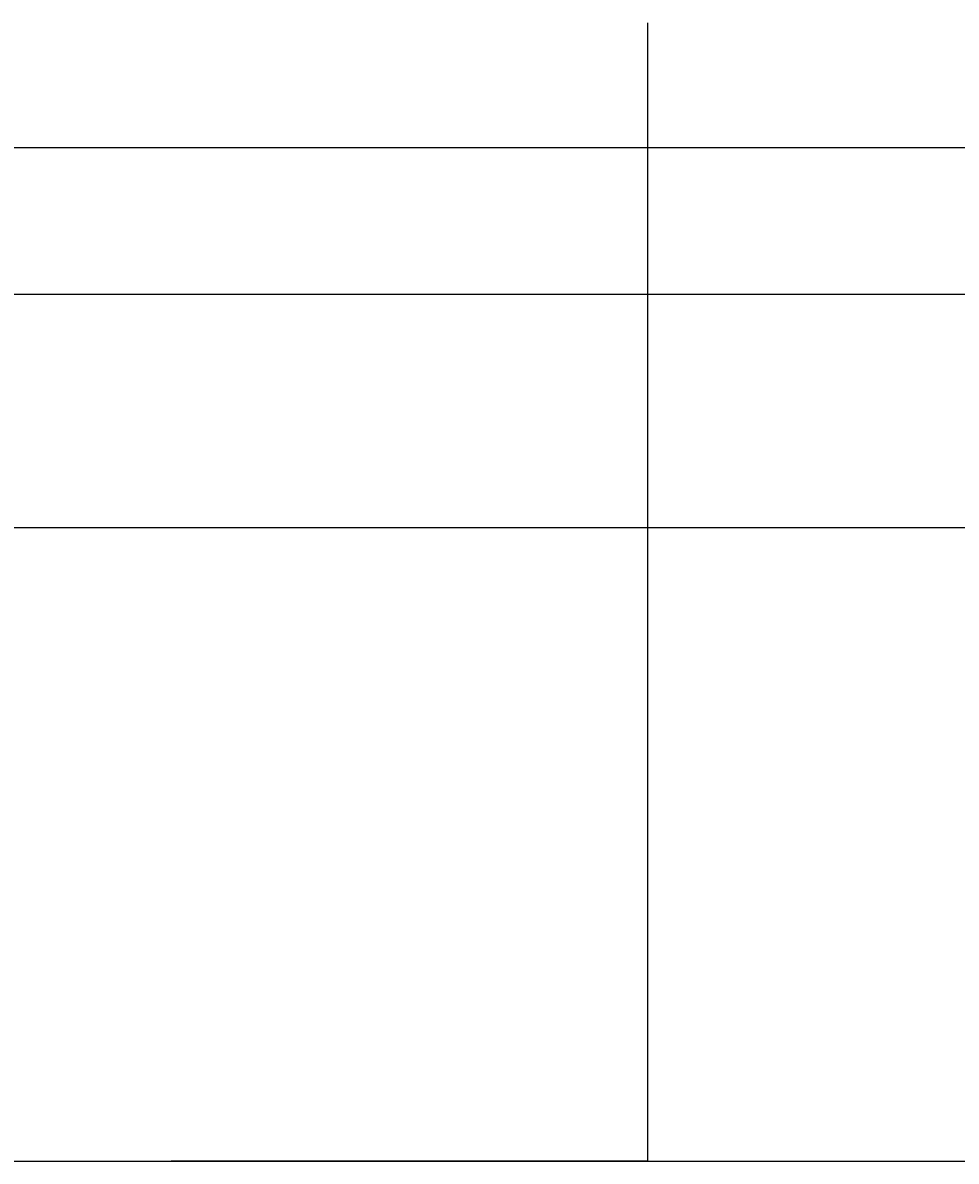
# Model space of a CAD drawing. Units: inches. Extents: x 35362 to 73946, y 43607 to 67532.
# Tile 2 of 134: x 38077 to 40793, y 43607 to 46919. Entities that reach past the tile are written whole.
import ezdxf

# ---------------------------------------------------------------- set-up
doc = ezdxf.new("R2010")
doc.units = ezdxf.units.IN
doc.header["$MEASUREMENT"] = 0
doc.layers.add('A-ANNO-DIMS', color=2, linetype='Continuous', lineweight=18)
doc.styles.get("Standard").update_dxf_attribs({"font": 'arial.ttf'})
doc.dimstyles.get("Standard").update_dxf_attribs({"dimtxt": 0.18, "dimasz": 0.18, "dimexe": 0.18, "dimexo": 0.0625, "dimgap": 0.09, "dimtad": 0, "dimtih": 1, "dimtoh": 1, "dimdec": 4, "dimzin": 0, "dimdsep": 46, "dimtxsty": 'Standard', "dimcen": 0.09, "dimadec": 0, "dimazin": 0, "dimtfac": 1, "dimtdec": 4, "dimtofl": 0, "dimtmove": 0, "dimatfit": 3, "dimfxl": 1, "dimtolj": 1, "dimtzin": 0, "dimarcsym": 0})

# ---------------------------------------------------------------- blocks, each defined once
blk = doc.blocks.new('*D5')
at = {"layer": 'A-ANNO-DIMS', "color": 0, "lineweight": -2, "transparency": 16777216}
for p, q in [((37121.9, 46919.3), (37121.9, 43606.7)), ((69871.5, 45449.8), (69871.5, 43606.7)), ((37122.1, 43606.9), (53496.3, 43606.9)), ((69871.3, 43606.9), (53497.2, 43606.9))]:
    blk.add_line(p, q, dxfattribs=at)
at = {"layer": 'A-ANNO-DIMS', "color": 0, "transparency": 16777216}
for points in [[(37122.1, 43606.9), (37122.1, 43606.8), (37121.9, 43606.9)], [(69871.3, 43606.9), (69871.3, 43606.8), (69871.5, 43606.9)]]:
    blk.add_solid(points, dxfattribs=at)
at = {"layer": 'Defpoints', "color": 0, "transparency": 16777216}
for p in [(37121.9, 46919.4), (69871.5, 45449.9), (69871.5, 43606.9)]:
    blk.add_point(p, dxfattribs=at)
at = {"layer": 'A-ANNO-DIMS', "color": 0, "transparency": 16777216, "insert": (53496.7, 43606.9), "char_height": 0.18, "attachment_point": 5}
blk.add_mtext('\\A1;32750', dxfattribs=at)
blk = doc.blocks.new('*D15')
at = {"layer": 'A-ANNO-DIMS', "color": 0, "lineweight": -2, "transparency": 16777216}
for p, q in [((37121.9, 46919.3), (37121.9, 43606.7)), ((39894.8, 46919.3), (39894.8, 43606.7)), ((37122.1, 43606.9), (38508, 43606.9)), ((39894.7, 43606.9), (38508.8, 43606.9))]:
    blk.add_line(p, q, dxfattribs=at)
at = {"layer": 'A-ANNO-DIMS', "color": 0, "transparency": 16777216}
for points in [[(37122.1, 43606.9), (37122.1, 43606.8), (37121.9, 43606.9)], [(39894.7, 43606.9), (39894.7, 43606.8), (39894.8, 43606.9)]]:
    blk.add_solid(points, dxfattribs=at)
at = {"layer": 'Defpoints', "color": 0, "transparency": 16777216}
for p in [(37121.9, 46919.4), (39894.8, 46919.4), (39894.8, 43606.9)]:
    blk.add_point(p, dxfattribs=at)
at = {"layer": 'A-ANNO-DIMS', "color": 0, "transparency": 16777216, "insert": (38508.4, 43606.9), "char_height": 0.18, "attachment_point": 5}
blk.add_mtext('\\A1;2773', dxfattribs=at)
blk = doc.blocks.new('*D41')
at = {"layer": 'A-ANNO-DIMS', "color": 0, "lineweight": -2, "transparency": 16777216}
for p, q in [((39894.8, 46919.3), (39894.8, 43606.7)), ((45390.1, 46919.3), (45390.1, 43606.7)), ((39895, 43606.9), (42642, 43606.9)), ((45390, 43606.9), (42643, 43606.9))]:
    blk.add_line(p, q, dxfattribs=at)
at = {"layer": 'A-ANNO-DIMS', "color": 0, "transparency": 16777216}
for points in [[(39895, 43606.9), (39895, 43606.8), (39894.8, 43606.9)], [(45390, 43606.9), (45390, 43606.8), (45390.1, 43606.9)]]:
    blk.add_solid(points, dxfattribs=at)
at = {"layer": 'Defpoints', "color": 0, "transparency": 16777216}
for p in [(39894.8, 46919.4), (45390.1, 46919.4), (45390.1, 43606.9)]:
    blk.add_point(p, dxfattribs=at)
at = {"layer": 'A-ANNO-DIMS', "color": 0, "transparency": 16777216, "insert": (42642.5, 43606.9), "char_height": 0.18, "attachment_point": 5}
blk.add_mtext('\\A1;5495.3', dxfattribs=at)
blk = doc.blocks.new('*D67')
at = {"layer": 'A-ANNO-DIMS', "color": 0, "lineweight": -2, "transparency": 16777216}
for p, q in [((56873.5, 53351.5), (35361.8, 53351.5)), ((35361.9, 53351.3), (35361.9, 49400.9)), ((35361.9, 45450.1), (35361.9, 49400.5)), ((53793.6, 45449.9), (35361.8, 45449.9))]:
    blk.add_line(p, q, dxfattribs=at)
at = {"layer": 'A-ANNO-DIMS', "color": 0, "transparency": 16777216}
for points in [[(35361.9, 53351.3), (35362, 53351.3), (35361.9, 53351.5)], [(35361.9, 45450.1), (35362, 45450.1), (35361.9, 45449.9)]]:
    blk.add_solid(points, dxfattribs=at)
at = {"layer": 'Defpoints', "color": 0, "transparency": 16777216}
for p in [(35361.9, 53351.5), (56873.6, 53351.5), (53793.6, 45449.9)]:
    blk.add_point(p, dxfattribs=at)
at = {"layer": 'A-ANNO-DIMS', "color": 0, "transparency": 16777216, "insert": (35361.9, 49400.7), "char_height": 0.18, "attachment_point": 5}
blk.add_mtext('\\A1;7901.6', dxfattribs=at)
blk = doc.blocks.new('*D76')
at = {"layer": 'A-ANNO-DIMS', "color": 0, "lineweight": -2, "transparency": 16777216}
for p, q in [((54052.8, 46555.3), (35361.8, 46555.3)), ((35361.9, 46555.1), (35361.9, 46342.3)), ((35361.9, 46129.1), (35361.9, 46341.9)), ((53793.6, 46128.9), (35361.8, 46128.9))]:
    blk.add_line(p, q, dxfattribs=at)
at = {"layer": 'A-ANNO-DIMS', "color": 0, "transparency": 16777216}
for points in [[(35361.9, 46555.1), (35362, 46555.1), (35361.9, 46555.3)], [(35361.9, 46129.1), (35362, 46129.1), (35361.9, 46128.9)]]:
    blk.add_solid(points, dxfattribs=at)
at = {"layer": 'Defpoints', "color": 0, "transparency": 16777216}
for p in [(35361.9, 46555.3), (54052.9, 46555.3), (53793.6, 46128.9)]:
    blk.add_point(p, dxfattribs=at)
at = {"layer": 'A-ANNO-DIMS', "color": 0, "transparency": 16777216, "insert": (35361.9, 46342.1), "char_height": 0.18, "attachment_point": 5}
blk.add_mtext('\\A1;426.4', dxfattribs=at)
blk = doc.blocks.new('*D90')
at = {"layer": 'A-ANNO-DIMS', "color": 0, "lineweight": -2, "transparency": 16777216}
for p, q in [((53707.7, 47291.3), (35361.8, 47291.3)), ((35361.9, 47291.1), (35361.9, 46710.3)), ((35361.9, 46129.1), (35361.9, 46709.9)), ((53793.6, 46128.9), (35361.8, 46128.9))]:
    blk.add_line(p, q, dxfattribs=at)
at = {"layer": 'A-ANNO-DIMS', "color": 0, "transparency": 16777216}
for points in [[(35361.9, 47291.1), (35362, 47291.1), (35361.9, 47291.3)], [(35361.9, 46129.1), (35362, 46129.1), (35361.9, 46128.9)]]:
    blk.add_solid(points, dxfattribs=at)
at = {"layer": 'Defpoints', "color": 0, "transparency": 16777216}
for p in [(53707.8, 47291.3), (35361.9, 46128.9), (53793.6, 46128.9)]:
    blk.add_point(p, dxfattribs=at)
at = {"layer": 'A-ANNO-DIMS', "color": 0, "transparency": 16777216, "insert": (35361.9, 46710.1), "char_height": 0.18, "attachment_point": 5}
blk.add_mtext('\\A1;1162.4', dxfattribs=at)

msp = doc.modelspace()

# ---------------------------------------------------------------- dimensions: what is measured, and where the dimension line sits
at = {"layer": 'A-ANNO-DIMS'}
for base, p1, p2, picture, middle in [((35361.949, 53351.529), (53793.638, 45449.894), (56873.602, 53351.529), '*D67', (35361.949, 49400.712)), ((35361.949, 46128.878), (53707.781, 47291.285), (53793.638, 46128.878), '*D90', (35361.949, 46710.081)), ((35361.949, 46555.293), (53793.638, 46128.878), (54052.899, 46555.293), '*D76', (35361.949, 46342.086))]:
    dim = msp.add_linear_dim(base=base, p1=p1, p2=p2, angle=90, dimstyle='Standard', override={"dimdec": 1, "dimlfac": 1, "dimrnd": 0, "dimzin": 0, "dimdsep": 46, "dimlunit": 2}, dxfattribs=at)
    dim.commit()
    dim.dimension.update_dxf_attribs({"geometry": picture, "text_midpoint": middle})
for base, p1, p2, override, picture, middle in [((69871.496, 43606.859), (37121.949, 46919.381), (69871.496, 45449.894), {"dimdec": 0, "dimlfac": 1, "dimrnd": 0, "dimzin": 0, "dimdsep": 46, "dimlunit": 2}, '*D5', (53496.723, 43606.859)), ((39894.84, 43606.859), (37121.949, 46919.381), (39894.84, 46919.381), {"dimdec": 0, "dimlfac": 1, "dimrnd": 0, "dimzin": 0, "dimdsep": 46, "dimlunit": 2}, '*D15', (38508.395, 43606.859)), ((45390.147, 43606.859), (39894.84, 46919.381), (45390.147, 46919.381), {"dimdec": 1, "dimlfac": 1, "dimrnd": 0, "dimzin": 0, "dimdsep": 46, "dimlunit": 2}, '*D41', (42642.494, 43606.859))]:
    dim = msp.add_linear_dim(base=base, p1=p1, p2=p2, dimstyle='Standard', override=override, dxfattribs=at)
    dim.commit()
    dim.dimension.update_dxf_attribs({"geometry": picture, "text_midpoint": middle})

doc.saveas('drawing.dxf')
